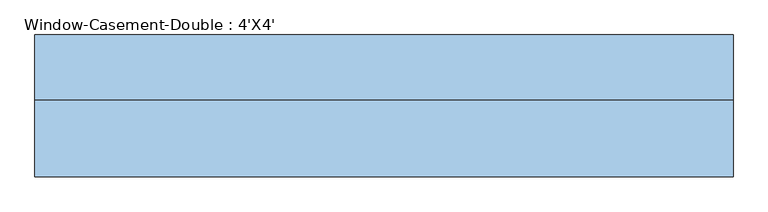
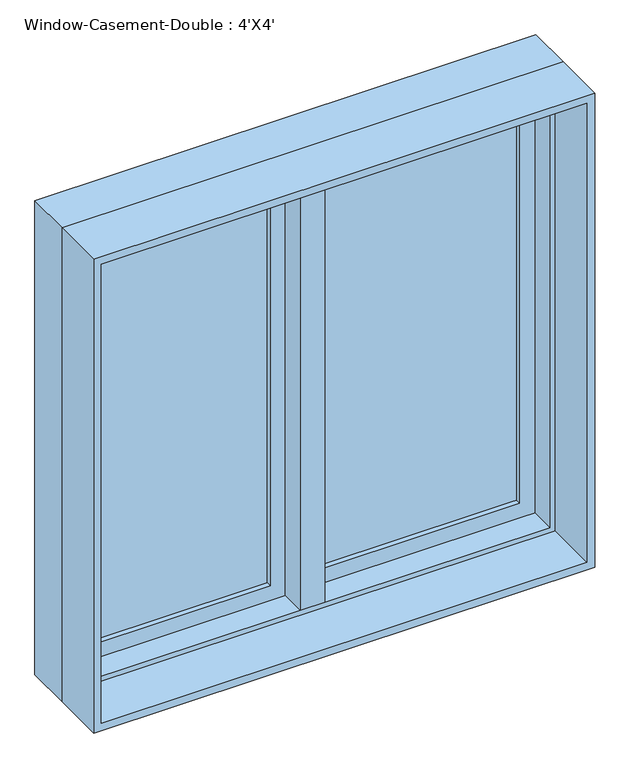
"""IFC4 building model written with IfcOpenShell, lengths in millimetres: window geometry, Window-Casement-Double : 4'X4'."""

from ifc_helpers import new_model, si_unit, frame, origin, place, context, project, spatial, polyline, outline, extrude, faceted_brep, source, transform, mapped, element, save


def window_casement_double_4_x4_af3140d2(model_context):
    return source(origin(), model_context, "Body", "SolidModel", [
        faceted_brep([(9.525, 133.35, 2120.9), (-9.525, 133.35, 2120.9), (-9.525, 82.55, 2120.9), (9.525, 82.55, 2120.9), (9.525, 133.35, 927.1), (9.525, 82.55, 927.1), (-9.525, 82.55, 927.1), (-9.525, 133.35, 927.1), (-9.525, 82.55, 946.15), (-9.525, 82.55, 2101.85), (-30.1625, 82.55, 946.15), (-30.1625, 82.55, 2101.85), (-30.1625, 19.05, 946.15), (-30.1625, 19.05, 2101.85), (30.1625, 19.05, 946.15), (30.1625, 19.05, 2101.85), (30.1625, 82.55, 946.15), (30.1625, 82.55, 2101.85), (9.525, 82.55, 946.15), (9.525, 82.55, 2101.85)], [[[0, 1, 2, 3]], [[4, 5, 6, 7]], [[1, 0, 4, 7]], [[2, 1, 7, 6, 8, 9]], [[9, 8, 10, 11]], [[11, 10, 12, 13]], [[13, 12, 14, 15]], [[15, 14, 16, 17]], [[17, 16, 18, 19]], [[0, 3, 19, 18, 5, 4]], [[18, 8, 6, 5]], [[9, 19, 3, 2]], [[8, 18, 16, 14, 12, 10]], [[19, 9, 11, 13, 15, 17]]]),
        extrude(outline(polyline([(-66.675, 114.3), (-66.675, 107.95), (-539.75, 107.95), (-539.75, 114.3), (-66.675, 114.3)])), frame((0.0, 0.0, 984.25), z_axis=(0.0, 0.0, 1.0), x_axis=(1.0, 0.0, 0.0)), (0.0, 0.0, 1.0), 1079.5),
        extrude(outline(polyline([(-539.75, 95.25), (-539.75, 101.6), (-66.675, 101.6), (-66.675, 95.25), (-539.75, 95.25)])), frame((0.0, 0.0, 984.25), z_axis=(0.0, 0.0, 1.0), x_axis=(1.0, 0.0, 0.0)), (0.0, 0.0, 1.0), 1079.5),
        extrude(outline(polyline([(539.75, 114.3), (539.75, 107.95), (66.675, 107.95), (66.675, 114.3), (539.75, 114.3)])), frame((0.0, 0.0, 984.25), z_axis=(0.0, 0.0, 1.0), x_axis=(1.0, 0.0, 0.0)), (0.0, 0.0, 1.0), 1079.5),
        extrude(outline(polyline([(66.675, 95.25), (66.675, 101.6), (539.75, 101.6), (539.75, 95.25), (66.675, 95.25)])), frame((0.0, 0.0, 984.25), z_axis=(0.0, 0.0, 1.0), x_axis=(1.0, 0.0, 0.0)), (0.0, 0.0, 1.0), 1079.5),
        extrude(outline(polyline([(2120.9, -596.9), (927.1, -596.9), (927.1, -9.525), (2120.9, -9.525), (2120.9, -596.9)]), holes=[polyline([(2063.75, -66.675), (984.25, -66.675), (984.25, -539.75), (2063.75, -539.75), (2063.75, -66.675)])]), frame((0.0, 82.55, 0.0), z_axis=(0.0, 1.0, 0.0), x_axis=(0.0, 0.0, 1.0)), (0.0, 0.0, 1.0), 44.45),
        extrude(outline(polyline([(927.1, 596.9), (2120.9, 596.9), (2120.9, 9.525), (927.1, 9.525), (927.1, 596.9)]), holes=[polyline([(984.25, 66.675), (2063.75, 66.675), (2063.75, 539.75), (984.25, 539.75), (984.25, 66.675)])]), frame((0.0, 82.55, 0.0), z_axis=(0.0, 1.0, 0.0), x_axis=(0.0, 0.0, 1.0)), (0.0, 0.0, 1.0), 44.45),
        extrude(outline(polyline([(2133.6, -609.6), (914.4, -609.6), (914.4, 609.6), (2133.6, 609.6), (2133.6, -609.6)]), holes=[polyline([(2114.55, 590.55), (933.45, 590.55), (933.45, -590.55), (2114.55, -590.55), (2114.55, 590.55)])]), frame((0.0, -114.3, 0.0), z_axis=(0.0, 1.0, 0.0), x_axis=(0.0, 0.0, 1.0)), (0.0, 0.0, 1.0), 133.35),
        faceted_brep([(577.85, 82.55, 2101.85), (577.85, 19.05, 2101.85), (-577.85, 19.05, 2101.85), (-577.85, 82.55, 2101.85), (596.9, 133.35, 2120.9), (596.9, 82.55, 2120.9), (-596.9, 82.55, 2120.9), (-596.9, 133.35, 2120.9), (609.6, 19.05, 2133.6), (609.6, 133.35, 2133.6), (-609.6, 133.35, 2133.6), (-609.6, 19.05, 2133.6), (-577.85, 19.05, 946.15), (-577.85, 82.55, 946.15), (-596.9, 82.55, 927.1), (-596.9, 133.35, 927.1), (-609.6, 133.35, 914.4), (-609.6, 19.05, 914.4), (577.85, 19.05, 946.15), (577.85, 82.55, 946.15), (596.9, 82.55, 927.1), (596.9, 133.35, 927.1), (609.6, 133.35, 914.4), (609.6, 19.05, 914.4)], [[[0, 1, 2, 3]], [[4, 5, 6, 7]], [[8, 9, 10, 11]], [[3, 2, 12, 13]], [[7, 6, 14, 15]], [[11, 10, 16, 17]], [[13, 12, 18, 19]], [[15, 14, 20, 21]], [[17, 16, 22, 23]], [[11, 17, 23, 8], [1, 18, 12, 2]], [[19, 18, 1, 0]], [[5, 20, 14, 6], [3, 13, 19, 0]], [[21, 20, 5, 4]], [[23, 22, 9, 8]], [[9, 22, 16, 10], [7, 15, 21, 4]]]),
    ])


if __name__ == "__main__":
    model = new_model("IFC4")
    model_context = context("Model", 3, world=origin())
    ifc_project = project(units=[si_unit("LENGTHUNIT", "METRE", prefix="MILLI")], contexts=[model_context])
    site = spatial("IfcSite", under=ifc_project)
    building = spatial("IfcBuilding", under=site)
    placement = place(None, origin())
    window_casement_double_4_x4_shape = window_casement_double_4_x4_af3140d2(model_context)
    element("IfcWindow", 1, ObjectType="Window-Casement-Double : 4'X4'", at=placement, inside=building, context=model_context, shape_type="MappedRepresentation", body=[
        mapped(window_casement_double_4_x4_shape, transform((0.0, 0.0, 0.0), x_axis=(1.0, 0.0, 0.0), y_axis=(0.0, 1.0, 0.0), z_axis=(0.0, 0.0, 1.0))),
    ])
    save(model, "model.ifc")

# Revit data of these elements
# Type "Window-Casement-Double : 4'X4'"
#   Type Mark = "20"
#   Fire Rating = "0.5h"
#   Assembly Code = "B2020100"
#   Analytic Construction = "Double glazing - domestic"
#   Frame Extension [instance default] = 0' - 0 1/4"
#   Window Inset [instance default] = 0' - 0"
#   Wall Thickness [instance default] = 0' - 6"
#   Interior Wall Closure [instance default] = 0' - 2 1/4"
#   Half Width = 2' - 0"
#   Visual Light Transmittance = 0.81
#   Thermal Resistance (R) = 1.8146 (h·ft²·°F)/BTU
#   Solar Heat Gain Coefficient = 0.76
#   Rough Width = 4' - 0 1/2"
#   Rough Height = 4' - 0 1/2"
#   Height = 4' - 0"
#   Heat Transfer Coefficient (U) = 0.5511 BTU/(h·ft²·°F)
#   Exterior Wall Closure [instance default] = 0' - 1 1/4"
#   Extension Jamb [instance default] = 0' - 2 1/4"
#   Default Sill Height = 3' - 0"
#   Width = 4' - 0"
#   Muntin Visibility = yes
#   Interior Trim Visibility [instance default] = yes
#   Exterior Trim Visibility [instance default] = yes
#   Extension Jamb Visibility [instance default] = yes
#   Interior Trim Material = Wood - Stained
#   Muntin Pattern = Muntin Pattern_2x2 : Muntin Pattern_2x2
#   Interior Trim = Trim-Window-Interior-Flat : Picture Frame
#   Interior Frame Material = Wood - Stained
#   Glass Panel Material = Glass
#   Exterior Trim Material = Clad - White
#   Exterior Trim = Trim-Window-Exterior-Flat : with Sill
#   Exterior Frame Material = Clad - White
#   Wall Closure = (empty or 0)
# Element 1 (IfcWindow, "Window-Casement-Double : 4'X4'")
#   Wall Thickness = 0' - 9"
#   Extension Jamb = 0' - 5 1/4"
#   Materials on its faces: "Wood - Stained", "Glass", "Clad - White"
# Materials
#   "Wood - Stained": class "Wood", colour RGB 224 178 126, transparency 0, Cost = 0
#   "Glass": class "Glass", colour RGB 0 128 192, transparency 0.75, Description = "Soda Lime Glass", Cost = 0
#   "Clad - White": class "Wood", colour RGB 242 242 238, transparency 0, Cost = 0
